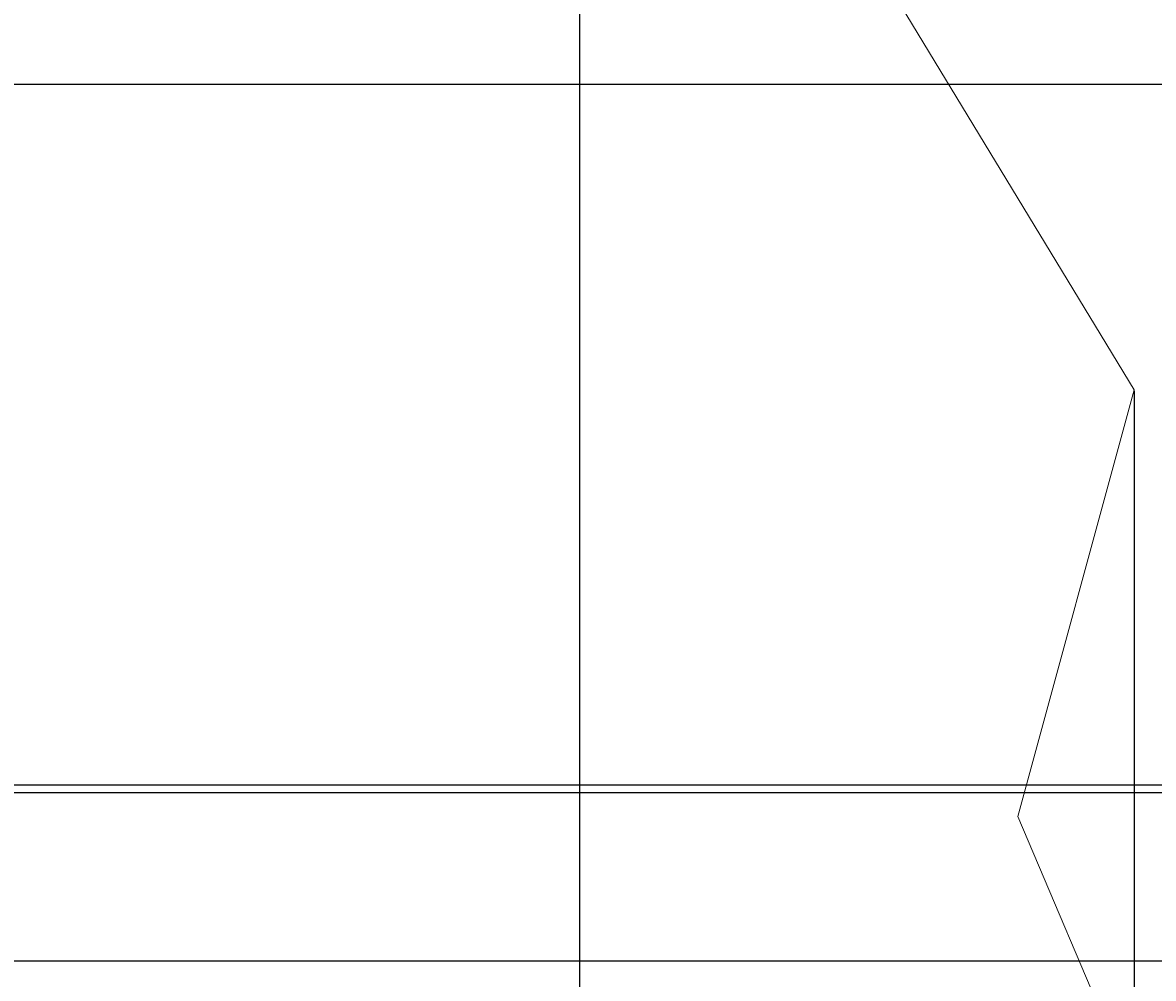
# Model space of a CAD drawing. Units: inches. Extents: x -26 to 776, y -22 to 650.
# Tile 49 of 62: x 506 to 586, y 158 to 226. Entities that reach past the tile are written whole.
import ezdxf

# ---------------------------------------------------------------- set-up
doc = ezdxf.new("R2010")
doc.units = ezdxf.units.IN
doc.header["$MEASUREMENT"] = 0
doc.layers.add('A-ANNO-DIMS', color=2, linetype='Continuous', lineweight=18)
doc.layers.add('L-PLNT-TREE', color=94, linetype='Continuous', lineweight=18)
doc.styles.get("Standard").update_dxf_attribs({"font": 'arial.ttf'})
doc.dimstyles.get("Standard").update_dxf_attribs({"dimtxt": 0.5625, "dimasz": 0.18, "dimexe": 0.18, "dimexo": 0.0625, "dimgap": 0.09, "dimtad": 0, "dimtih": 1, "dimtoh": 1, "dimdec": 4, "dimzin": 0, "dimdsep": 46, "dimlunit": 4, "dimtxsty": 'Standard', "dimcen": 0.09, "dimadec": 0, "dimazin": 0, "dimtfac": 1, "dimtdec": 4, "dimtofl": 0, "dimtmove": 0, "dimatfit": 3, "dimfxl": 1, "dimtolj": 1, "dimtzin": 0, "dimarcsym": 0})

# ---------------------------------------------------------------- blocks, each defined once
blk = doc.blocks.new('Tree - type 2 deciduous elevation')
blk.add_lwpolyline([(19.675, 39.077), (23.701, 44.975), (30.027, 47.924), (30.602, 53.823), (25.426, 56.772), (32.903, 61.196), (34.053, 67.094), (30.602, 75.205), (34.628, 89.951), (26.576, 103.222)])
blk = doc.blocks.new('*D20')
at = {"layer": 'A-ANNO-DIMS', "color": 0, "lineweight": -2, "transparency": 16777216}
for p, q in [((425.806, 455.472), (775.335, 455.472)), ((775.155, 455.292), (775.155, 235.854)), ((775.155, 15.662), (775.155, 235.1)), ((425.806, 15.482), (775.335, 15.482))]:
    blk.add_line(p, q, dxfattribs=at)
at = {"layer": 'A-ANNO-DIMS', "color": 0, "transparency": 16777216}
for points in [[(775.125, 455.292), (775.185, 455.292), (775.155, 455.472)], [(775.125, 15.662), (775.185, 15.662), (775.155, 15.482)]]:
    blk.add_solid(points, dxfattribs=at)
at = {"layer": 'Defpoints', "color": 0, "transparency": 16777216}
for p in [(425.743, 455.472), (775.155, 455.472), (425.743, 15.482)]:
    blk.add_point(p, dxfattribs=at)
at = {"layer": 'A-ANNO-DIMS', "color": 0, "transparency": 16777216, "insert": (775.155, 235.477), "char_height": 0.5625, "attachment_point": 5}
blk.add_mtext('\\A1;440', dxfattribs=at)
blk = doc.blocks.new('*D26')
at = {"layer": 'A-ANNO-DIMS', "color": 0, "lineweight": -2, "transparency": 16777216}
for p, q in [((91.707, 171.973), (775.335, 171.973)), ((775.155, 171.793), (775.155, 166.105)), ((775.155, 159.662), (775.155, 165.351)), ((82.196, 159.482), (775.335, 159.482))]:
    blk.add_line(p, q, dxfattribs=at)
at = {"layer": 'A-ANNO-DIMS', "color": 0, "transparency": 16777216}
for points in [[(775.125, 171.793), (775.185, 171.793), (775.155, 171.973)], [(775.125, 159.662), (775.185, 159.662), (775.155, 159.482)]]:
    blk.add_solid(points, dxfattribs=at)
at = {"layer": 'Defpoints', "color": 0, "transparency": 16777216}
for p in [(91.645, 171.973), (775.155, 171.973), (82.134, 159.482)]:
    blk.add_point(p, dxfattribs=at)
at = {"layer": 'A-ANNO-DIMS', "color": 0, "transparency": 16777216, "insert": (775.155, 165.728), "char_height": 0.5625, "attachment_point": 5}
blk.add_mtext('\\A1;12.49', dxfattribs=at)
blk = doc.blocks.new('*D28')
at = {"layer": 'A-ANNO-DIMS', "color": 0, "lineweight": -2, "transparency": 16777216}
for p, q in [((285.08, 314.119), (775.335, 314.119)), ((775.155, 313.939), (775.155, 243.141)), ((775.155, 171.597), (775.155, 242.396)), ((285.08, 171.417), (775.335, 171.417))]:
    blk.add_line(p, q, dxfattribs=at)
at = {"layer": 'A-ANNO-DIMS', "color": 0, "transparency": 16777216}
for points in [[(775.125, 313.939), (775.185, 313.939), (775.155, 314.119)], [(775.125, 171.597), (775.185, 171.597), (775.155, 171.417)]]:
    blk.add_solid(points, dxfattribs=at)
at = {"layer": 'Defpoints', "color": 0, "transparency": 16777216}
for p in [(285.018, 314.119), (775.155, 314.119), (285.018, 171.417)]:
    blk.add_point(p, dxfattribs=at)
at = {"layer": 'A-ANNO-DIMS', "color": 0, "transparency": 16777216, "insert": (775.155, 242.768), "char_height": 0.5625, "attachment_point": 5}
blk.add_mtext('\\A1;142.7', dxfattribs=at)
blk = doc.blocks.new('*D41')
at = {"layer": 'A-ANNO-DIMS', "color": 0, "lineweight": -2, "transparency": 16777216}
for p, q in [((11.17, 221.641), (775.335, 221.641)), ((775.155, 221.461), (775.155, 190.939)), ((775.155, 159.662), (775.155, 190.185)), ((11.17, 159.482), (775.335, 159.482))]:
    blk.add_line(p, q, dxfattribs=at)
at = {"layer": 'A-ANNO-DIMS', "color": 0, "transparency": 16777216}
for points in [[(775.125, 221.461), (775.185, 221.461), (775.155, 221.641)], [(775.125, 159.662), (775.185, 159.662), (775.155, 159.482)]]:
    blk.add_solid(points, dxfattribs=at)
at = {"layer": 'Defpoints', "color": 0, "transparency": 16777216}
for p in [(11.107, 221.641), (775.155, 221.641), (11.107, 159.482)]:
    blk.add_point(p, dxfattribs=at)
at = {"layer": 'A-ANNO-DIMS', "color": 0, "transparency": 16777216, "insert": (775.155, 190.562), "char_height": 0.5625, "attachment_point": 5}
blk.add_mtext('\\A1;62.16', dxfattribs=at)
blk = doc.blocks.new('*D42')
at = {"layer": 'A-ANNO-DIMS', "color": 0, "lineweight": -2, "transparency": 16777216}
for p, q in [((285.08, 171.417), (775.335, 171.417)), ((775.155, 171.237), (775.155, 165.827)), ((775.155, 159.662), (775.155, 165.072)), ((289.305, 159.482), (775.335, 159.482))]:
    blk.add_line(p, q, dxfattribs=at)
at = {"layer": 'A-ANNO-DIMS', "color": 0, "transparency": 16777216}
for points in [[(775.125, 171.237), (775.185, 171.237), (775.155, 171.417)], [(775.125, 159.662), (775.185, 159.662), (775.155, 159.482)]]:
    blk.add_solid(points, dxfattribs=at)
at = {"layer": 'Defpoints', "color": 0, "transparency": 16777216}
for p in [(285.018, 171.417), (775.155, 171.417), (289.242, 159.482)]:
    blk.add_point(p, dxfattribs=at)
at = {"layer": 'A-ANNO-DIMS', "color": 0, "transparency": 16777216, "insert": (775.155, 165.45), "char_height": 0.5625, "attachment_point": 5}
blk.add_mtext('\\A1;11.935', dxfattribs=at)
blk = doc.blocks.new('*D45')
at = {"layer": 'A-ANNO-DIMS', "color": 0, "lineweight": -2, "transparency": 16777216}
for p, q in [((507.738, 408.639), (775.335, 408.639)), ((775.155, 408.459), (775.155, 212.438)), ((775.155, 15.662), (775.155, 211.683)), ((585.998, 15.482), (775.335, 15.482))]:
    blk.add_line(p, q, dxfattribs=at)
at = {"layer": 'A-ANNO-DIMS', "color": 0, "transparency": 16777216}
for points in [[(775.125, 408.459), (775.185, 408.459), (775.155, 408.639)], [(775.125, 15.662), (775.185, 15.662), (775.155, 15.482)]]:
    blk.add_solid(points, dxfattribs=at)
at = {"layer": 'Defpoints', "color": 0, "transparency": 16777216}
for p in [(507.676, 408.639), (775.155, 408.639), (585.935, 15.482)]:
    blk.add_point(p, dxfattribs=at)
at = {"layer": 'A-ANNO-DIMS', "color": 0, "transparency": 16777216, "insert": (775.155, 212.061), "char_height": 0.5625, "attachment_point": 5}
blk.add_mtext('\\A1;393.16', dxfattribs=at)
blk = doc.blocks.new('*D47')
at = {"layer": 'A-ANNO-DIMS', "color": 0, "lineweight": -2, "transparency": 16777216}
for p, q in [((584.343, 199.901), (584.343, -21.315)), ((428.648, 180.243), (428.648, -21.315)), ((428.828, -21.135), (505.483, -21.135)), ((584.163, -21.135), (507.508, -21.135))]:
    blk.add_line(p, q, dxfattribs=at)
at = {"layer": 'A-ANNO-DIMS', "color": 0, "transparency": 16777216}
for points in [[(428.828, -21.105), (428.828, -21.165), (428.648, -21.135)], [(584.163, -21.105), (584.163, -21.165), (584.343, -21.135)]]:
    blk.add_solid(points, dxfattribs=at)
at = {"layer": 'Defpoints', "color": 0, "transparency": 16777216}
for p in [(584.343, 199.963), (428.648, 180.305), (584.343, -21.135)]:
    blk.add_point(p, dxfattribs=at)
at = {"layer": 'A-ANNO-DIMS', "color": 0, "transparency": 16777216, "insert": (506.496, -21.135), "char_height": 0.5625, "attachment_point": 5}
blk.add_mtext('\\A1;155.7', dxfattribs=at)
blk = doc.blocks.new('*D48')
at = {"layer": 'A-ANNO-DIMS', "color": 0, "lineweight": -2, "transparency": 16777216}
for p, q in [((545.033, 67.415), (545.033, 649.856)), ((545.213, 649.676), (640.879, 649.676)), ((738.57, 649.676), (642.904, 649.676)), ((738.75, 50.911), (738.75, 649.856))]:
    blk.add_line(p, q, dxfattribs=at)
at = {"layer": 'A-ANNO-DIMS', "color": 0, "transparency": 16777216}
for points in [[(545.213, 649.706), (545.213, 649.646), (545.033, 649.676)], [(738.57, 649.706), (738.57, 649.646), (738.75, 649.676)]]:
    blk.add_solid(points, dxfattribs=at)
at = {"layer": 'Defpoints', "color": 0, "transparency": 16777216}
for p in [(738.75, 649.676), (545.033, 67.352), (738.75, 50.848)]:
    blk.add_point(p, dxfattribs=at)
at = {"layer": 'A-ANNO-DIMS', "color": 0, "transparency": 16777216, "insert": (641.892, 649.676), "char_height": 0.5625, "attachment_point": 5}
blk.add_mtext('\\A1;193.7', dxfattribs=at)

msp = doc.modelspace()

# ---------------------------------------------------------------- block references
at = {"layer": 'L-PLNT-TREE', "xscale": 2.050905272406618, "yscale": 2.050905272406618, "zscale": 2.050905272406618}
msp.add_blockref('Tree - type 2 deciduous elevation', (513.3241, 15.4824), dxfattribs=at)

# ---------------------------------------------------------------- dimensions: what is measured, and where the dimension line sits
at = {"layer": 'A-ANNO-DIMS'}
for base, p1, p2, picture, middle in [((738.7503, 649.6763), (545.0331, 67.3523), (738.7503, 50.8482), '*D48', (641.8917, 649.6763)), ((584.3428, -21.1349), (428.6484, 180.3054), (584.3428, 199.9634), '*D47', (506.4956, -21.1349))]:
    dim = msp.add_linear_dim(base=base, p1=p1, p2=p2, dimstyle='Standard', override={"dimdec": 1, "dimlfac": 1, "dimrnd": 0, "dimzin": 0, "dimdsep": 46, "dimlunit": 2}, dxfattribs=at)
    dim.commit()
    dim.dimension.update_dxf_attribs({"geometry": picture, "text_midpoint": middle})
for base, p1, p2, override, picture, middle in [((775.1553, 455.4717), (425.7434, 15.4824), (425.7434, 455.4717), {"dimdec": 0, "dimlfac": 1, "dimrnd": 0, "dimzin": 0, "dimdsep": 46, "dimlunit": 2}, '*D20', (775.1553, 235.477)), ((775.1553, 408.6389), (585.9354, 15.4824), (507.6759, 408.6389), {"dimdec": 2, "dimlfac": 1, "dimrnd": 0, "dimzin": 0, "dimdsep": 46, "dimlunit": 2}, '*D45', (775.1553, 212.0606)), ((775.1553, 314.119), (285.0179, 171.4173), (285.0179, 314.119), {"dimdec": 1, "dimlfac": 1, "dimrnd": 0, "dimzin": 0, "dimdsep": 46, "dimlunit": 2}, '*D28', (775.1553, 242.7682)), ((775.1553, 221.6413), (11.1074, 159.4824), (11.1074, 221.6413), {"dimdec": 2, "dimlfac": 1, "dimrnd": 0, "dimzin": 0, "dimdsep": 46, "dimlunit": 2}, '*D41', (775.1553, 190.5618)), ((775.1553, 171.9734), (82.134, 159.4824), (91.6448, 171.9734), {"dimdec": 2, "dimlfac": 1, "dimrnd": 0, "dimzin": 0, "dimdsep": 46, "dimlunit": 2}, '*D26', (775.1553, 165.7279)), ((775.1553, 171.4173), (289.2424, 159.4824), (285.0179, 171.4173), {"dimdec": 3, "dimlfac": 1, "dimrnd": 0, "dimzin": 0, "dimdsep": 46, "dimlunit": 2}, '*D42', (775.1553, 165.4498))]:
    dim = msp.add_linear_dim(base=base, p1=p1, p2=p2, angle=90, dimstyle='Standard', override=override, dxfattribs=at)
    dim.commit()
    dim.dimension.update_dxf_attribs({"geometry": picture, "text_midpoint": middle})

doc.saveas('drawing.dxf')
